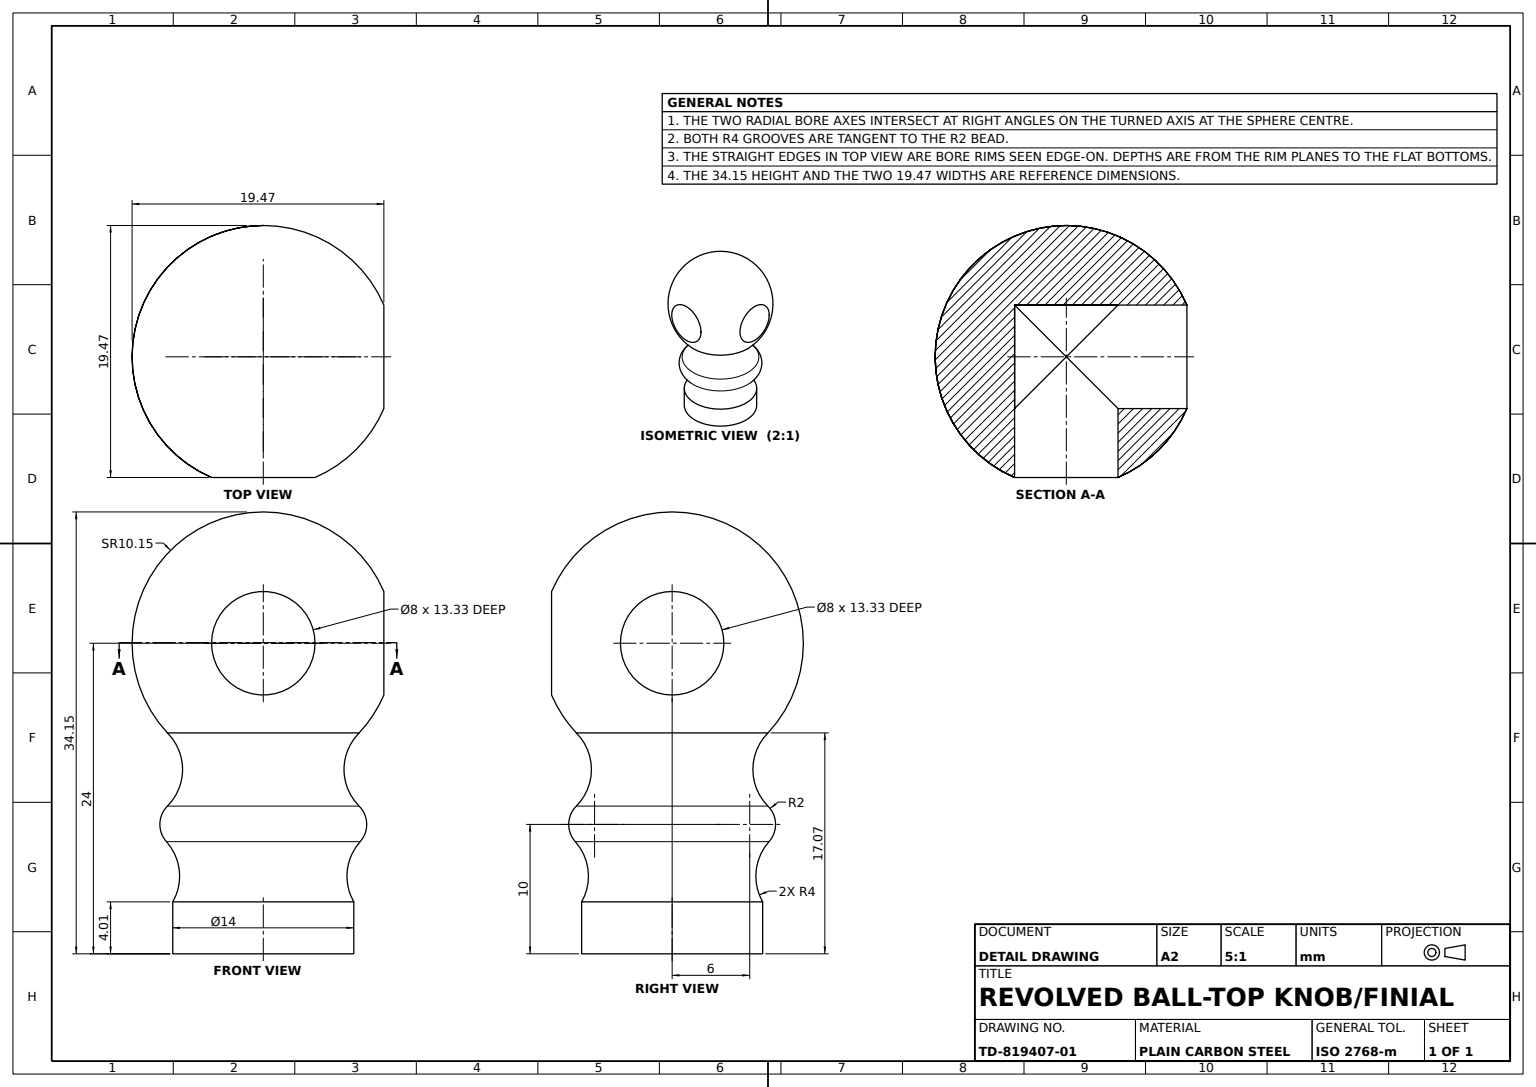
SolidWorks part; units mm, degrees
material "Plain Carbon Steel"
ref_plane "Front Plane" through (0, 0, 0) normal (0, 0, 1) x (1, 0, 0)
ref_plane "Top Plane" through (0, 0, 0) normal (0, 1, 0) x (1, 0, 0)
ref_plane "Right Plane" through (0, 0, 0) normal (1, 0, 0) x (0, 0, -1)
sketch "Knob Profile Sketch" plane through (0, 0, 0) normal (0, 0, 1) x (1, 0, 0)
  line L0 (0, 0) -> (0, 34.1479)
  line L1 (0, 0) -> (7, 0)
  line L4 (7, 0) -> (7, 4.014)
  line L6 (0, 0) -> (0, 24)
  arc A0 (7, 4.014) -> (7.4907, 8.6667) centre (10.4721, 6) cw
  arc A1 (7.4907, 8.6667) -> (7.4142, 11.4142) centre (6, 10) ccw
  arc A2 (7.4142, 11.4142) -> (7.4142, 17.0711) centre (10.2426, 14.2426) cw
  arc A3 (7.2804, 16.9306) -> (0, 34.1479) centre (0, 24) ccw
  dimension "D4" = 4
  dimension "D6" = 4
  dimension "D8" = 10.1479
  dimension "D5" = 2
  dimension "D1" = 7
  dimension "D2" = 6
  dimension "D3" = 10
  dimension "D7" = 6
  dimension "D9" = 7.2804
revolve "Knob Body Revolve" add sketch "Knob Profile Sketch" angle 360 about L0
sketch "Side Cut A Ø8 Sketch" plane through (0, 0, 0) normal (0, 0, 1) x (1, 0, 0)
  circle A0 centre (0, 24) radius 4
  dimension "D1" = 8
  dimension "D2" = 24
extrude "Side Cut A Ø8" cut sketch "Side Cut A Ø8 Sketch" against normal blind 14 and the other way blind 4
sketch "Side Cut B Ø8 Sketch" plane through (0, 0, 0) normal (1, 0, 0) x (0, 0, -1)
  circle A0 centre (0, 24) radius 4
  dimension "D1" = 8
  dimension "D2" = 24
extrude "Side Cut B Ø8" cut sketch "Side Cut B Ø8 Sketch" against normal blind 14 and the other way blind 4
